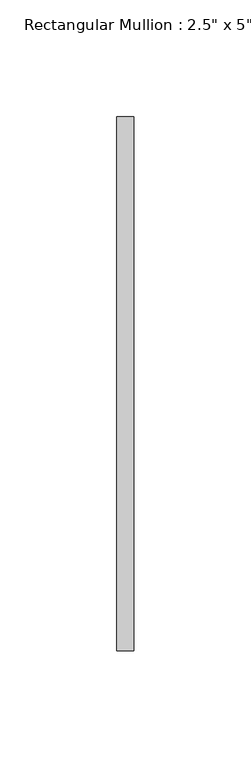
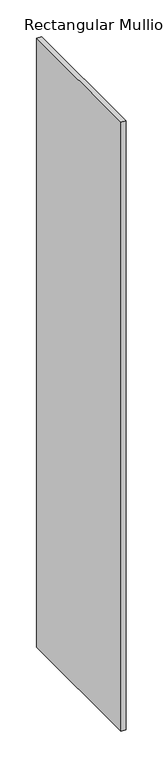
"""IFC4 building model written with IfcOpenShell, lengths in millimetres: member geometry."""

from ifc_helpers import new_model, si_unit, frame, origin, place, context, project, spatial, polyline, outline, extrude, source, transform, mapped, element, save


def member_781c77f6(model_context):
    return source(origin(), model_context, "Body", "SweptSolid", [
        extrude(outline(polyline([(3.6195, 114.3), (3.6195, -114.3), (-3.6195, -114.3), (-3.6195, 114.3), (3.6195, 114.3)])), frame((0.0, 0.0, -1005.1415), z_axis=(0.0, 0.0, 1.0), x_axis=(1.0, 0.0, 0.0)), (0.0, 0.0, 1.0), 1005.1415),
    ])


if __name__ == "__main__":
    model = new_model("IFC4")
    model_context = context("Model", 3, world=origin())
    ifc_project = project(units=[si_unit("LENGTHUNIT", "METRE", prefix="MILLI")], contexts=[model_context])
    site = spatial("IfcSite", under=ifc_project)
    building = spatial("IfcBuilding", under=site)
    placement = place(None, origin())
    member_shape = member_781c77f6(model_context)
    element("IfcMember", 1, ObjectType="Rectangular Mullion : 2.5\" x 5\" rectangular", at=placement, inside=building, context=model_context, shape_type="MappedRepresentation", body=[
        mapped(member_shape, transform((0.0, 0.0, 0.0), x_axis=(1.0, 0.0, 0.0), y_axis=(0.0, 1.0, 0.0), z_axis=(0.0, 0.0, 1.0))),
    ])
    save(model, "model.ifc")

# Revit data of these elements
# Type "Rectangular Mullion : 2.5\" x 5\" rectangular"
#   built-in parameter 1007304 = 0.75 (stored number, unit not read)
#   built-in parameter 1007301 = 0.011875 (stored number, unit not read)
#   built-in parameter 1007300 = 0.011875 (stored number, unit not read)
# Element 1 (IfcMember, "Rectangular Mullion : 2.5\" x 5\" rectangular")
#   Materials on its faces: "WINDOW GLASS MATERIAL"
# Materials
#   "WINDOW GLASS MATERIAL": class "Generic", colour RGB 120 120 120, transparency 0, Cost = 0
